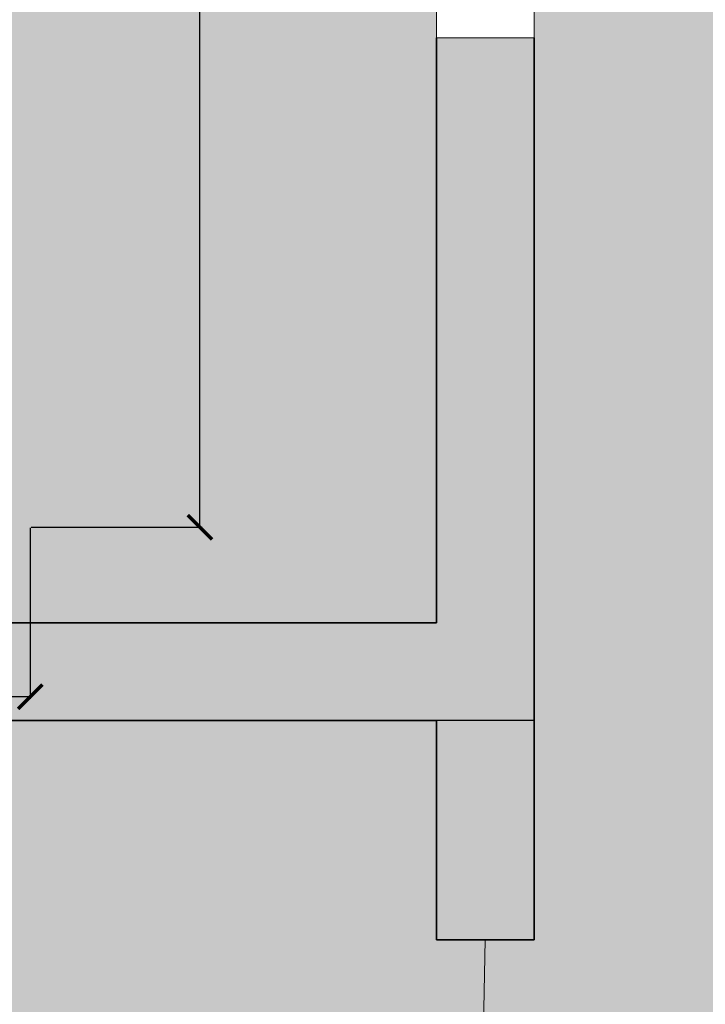
# Model space of a CAD drawing. Units: inches. Extents: x 1704 to 6393, y -157 to 1172.
# Tile 35 of 122: x 2563 to 2619, y 67 to 148. Entities that reach past the tile are written whole.
import ezdxf

# ---------------------------------------------------------------- set-up
doc = ezdxf.new("R2010")
doc.units = ezdxf.units.IN
doc.header["$MEASUREMENT"] = 0
for name, color, linetype, lineweight in [('A-ANNO-DIMS', 7, 'Continuous', 13), ('A-WALL-PATT', 7, 'Continuous', 13), ('L-HRDS', 8, 'Continuous', 18), ('L-PVMT-PATT', 8, 'Continuous', 13), ('WALLS', 7, 'Continuous', 35), ('WINDOWS', 2, 'Continuous', 18)]:
    doc.layers.add(name, color=color, linetype=linetype, lineweight=lineweight)
doc.layers.add('A-FLOR-PATT', color=7, linetype='Continuous', lineweight=13, true_color=0xf2f2f2)
doc.layers.add('L-HRDS-PATT', color=9, linetype='Continuous', lineweight=13, true_color=0xc5c1ba)
doc.styles.get("Standard").update_dxf_attribs({"font": 'arial.ttf'})
doc.dimstyles.get("Standard").update_dxf_attribs({"dimtxt": 6, "dimasz": 2, "dimexe": 0.18, "dimexo": 0.0625, "dimgap": 0.09, "dimtad": 0, "dimtih": 1, "dimtoh": 1, "dimdec": 1, "dimzin": 0, "dimdsep": 46, "dimlunit": 3, "dimtxsty": 'Standard', "dimblk": 'ARCHTICK', "dimcen": 0.09, "dimadec": 0, "dimazin": 0, "dimtfac": 1, "dimtdec": 1, "dimtofl": 0, "dimtmove": 0, "dimatfit": 3, "dimfxl": 1, "dimtolj": 1, "dimtzin": 0, "dimarcsym": 0})

# ---------------------------------------------------------------- blocks, each defined once
blk = doc.blocks.new('WIN-SLIDER-72')
for p, q in [((0, 72), (0, 0)), ((0, 72), (8, 72)), ((8, 66.251), (8, 72)), ((0, 67.227), (8, 67.227)), ((1.169, 36), (1.169, 64.3)), ((8, 7.7), (8, 64.3)), ((3.12, 37.952), (3.12, 62.348)), ((4.096, 37.952), (4.096, 62.348)), ((5.072, 37.952), (5.072, 62.348)), ((2.144, 37.952), (2.144, 42.144)), ((5.072, 36), (5.072, 7.7)), ((1.169, 9.652), (1.169, 34.048)), ((2.144, 9.652), (2.144, 34.048)), ((3.12, 9.652), (3.12, 34.048)), ((4.096, 34.048), (4.096, 29.856)), ((8, 5.749), (8, 0)), ((0, 4.773), (8, 4.773)), ((0, 0), (8, 0))]:
    blk.add_line(p, q)
for points in [[(8, 64.3), (8, 66.251), (0, 66.251), (0, 64.3)], [(5.072, 62.348), (5.072, 64.3), (3.12, 64.3), (3.12, 62.348)], [(2.144, 42.649), (1.853, 42.144), (2.436, 42.144)], [(5.072, 36), (5.072, 37.952), (3.12, 37.952), (3.12, 36)], [(3.12, 34.048), (3.12, 36), (1.169, 36), (1.169, 34.048)], [(4.096, 29.351), (3.804, 29.856), (4.388, 29.856)], [(3.12, 7.7), (3.12, 9.652), (1.169, 9.652), (1.169, 7.7)], [(8, 7.7), (8, 5.749), (0, 5.749), (0, 7.7)]]:
    blk.add_lwpolyline(points, close=True)
blk = doc.blocks.new('_ArchTick')
at = {"color": 0, "linetype": 'ByBlock', "const_width": 0.15}
blk.add_lwpolyline([(-0.5, -0.5), (0.5, 0.5)], dxfattribs=at)
blk = doc.blocks.new('*D64')
at = {"layer": 'A-ANNO-DIMS', "color": 0, "lineweight": -2, "transparency": 16777216}
for p, q in [((2564.089, 198.786), (2578.115, 198.786)), ((2577.935, 198.786), (2577.935, 155.58)), ((2577.935, 106.063), (2577.935, 149.269)), ((2564.089, 106.063), (2578.115, 106.063))]:
    blk.add_line(p, q, dxfattribs=at)
at = {"layer": 'Defpoints', "color": 0, "lineweight": -3, "transparency": 16777216}
for p in [(2564.026, 198.786), (2564.026, 106.063), (2577.935, 106.063)]:
    blk.add_point(p, dxfattribs=at)
at = {"layer": 'A-ANNO-DIMS', "color": 0, "lineweight": -2, "transparency": 16777216, "xscale": 2, "yscale": 2, "zscale": 2}
for p, rotation in [((2577.935, 198.786), 90), ((2577.935, 106.063), 270)]:
    blk.add_blockref('_ArchTick', p, dxfattribs=dict(at, rotation=rotation))
at = {"layer": 'A-ANNO-DIMS', "color": 0, "transparency": 16777216, "insert": (2577.935, 152.424), "char_height": 6, "attachment_point": 5}
blk.add_mtext('\\A1;BED 93', dxfattribs=at)
blk = doc.blocks.new('*D65')
at = {"layer": 'A-ANNO-DIMS', "color": 0, "lineweight": -2, "transparency": 16777216}
for p, q in [((2491.351, 106), (2491.351, 91.974)), ((2564.026, 106), (2564.026, 91.974)), ((2491.351, 92.154), (2523.326, 92.154)), ((2564.026, 92.154), (2532.051, 92.154))]:
    blk.add_line(p, q, dxfattribs=at)
at = {"layer": 'Defpoints', "color": 0, "lineweight": -3, "transparency": 16777216}
for p in [(2491.351, 106.063), (2564.026, 106.063), (2491.351, 92.154)]:
    blk.add_point(p, dxfattribs=at)
at = {"layer": 'A-ANNO-DIMS', "color": 0, "lineweight": -2, "transparency": 16777216, "xscale": 2, "yscale": 2, "zscale": 2, "rotation": 180}
blk.add_blockref('_ArchTick', (2491.351, 92.154), dxfattribs=at)
at = {"layer": 'A-ANNO-DIMS', "color": 0, "lineweight": -2, "transparency": 16777216, "xscale": 2, "yscale": 2, "zscale": 2}
blk.add_blockref('_ArchTick', (2564.026, 92.154), dxfattribs=at)
at = {"layer": 'A-ANNO-DIMS', "color": 0, "transparency": 16777216, "insert": (2527.689, 92.154), "char_height": 6, "attachment_point": 5}
blk.add_mtext('\\A1;73', dxfattribs=at)
blk = doc.blocks.new('*D93')
at = {"layer": 'A-ANNO-DIMS', "color": 0, "lineweight": -2, "transparency": 16777216}
for p, q in [((2605.286, 895.213), (1829.698, 895.213)), ((1829.878, 895.213), (1829.878, 495.866)), ((1829.878, 90.213), (1829.878, 489.56)), ((2605.286, 90.213), (1829.698, 90.213))]:
    blk.add_line(p, q, dxfattribs=at)
at = {"layer": 'Defpoints', "color": 0, "lineweight": -3, "transparency": 16777216}
for p in [(2605.349, 895.213), (1829.878, 90.213), (2605.349, 90.213)]:
    blk.add_point(p, dxfattribs=at)
at = {"layer": 'A-ANNO-DIMS', "color": 0, "lineweight": -2, "transparency": 16777216, "xscale": 2, "yscale": 2, "zscale": 2}
for p, rotation in [((1829.878, 895.213), 90), ((1829.878, 90.213), 270)]:
    blk.add_blockref('_ArchTick', p, dxfattribs=dict(at, rotation=rotation))
at = {"layer": 'A-ANNO-DIMS', "color": 0, "transparency": 16777216, "insert": (1829.878, 492.713), "char_height": 6, "attachment_point": 5}
blk.add_mtext('\\A1;805', dxfattribs=at)

msp = doc.modelspace()

# ---------------------------------------------------------------- hatches: boundary and pattern name
at = {"layer": 'A-FLOR-PATT', "transparency": 33554528}
h = msp.add_hatch(color=256, dxfattribs=at)
h.dxf.hatch_style = 1
h.paths.add_polyline_path([(2325.349, 863.213), (2325.349, 887.213), (2263.349, 887.213), (2167.349, 887.213), (2081.349, 887.213), (2081.349, 719.213), (2277.349, 719.213), (2277.349, 711.213), (2277.349, 372.213), (2349.349, 372.213), (2381.349, 372.213), (2381.349, 364.213), (2353.349, 364.213), (2353.349, 270.213), (2381.349, 270.213), (2381.349, 266.213), (2357.349, 266.213), (2357.349, 98.213), (2381.349, 98.213), (2385.181, 98.213), (2386.482, 98.213), (2424.215, 98.213), (2425.516, 98.213), (2429.349, 98.213), (2597.349, 98.213), (2597.349, 146.213), (2597.349, 218.213), (2597.349, 266.213), (2423.349, 266.213), (2423.349, 270.213), (2473.349, 270.213), (2473.349, 294.213), (2477.349, 294.213), (2477.349, 270.213), (2547.349, 270.213), (2547.349, 364.213), (2477.349, 364.213), (2477.349, 318.213), (2473.349, 318.213), (2473.349, 364.213), (2423.349, 364.213), (2423.349, 372.213), (2469.349, 372.213), (2469.349, 459.213), (2469.349, 538.213), (2350.349, 538.213), (2350.349, 565.713), (2358.349, 565.713), (2358.349, 545.213), (2420.349, 545.213), (2420.349, 610.213), (2358.349, 610.213), (2358.349, 589.713), (2350.349, 589.713), (2350.349, 615.213), (2425.349, 615.213), (2425.349, 607.213), (2425.349, 546.213), (2469.349, 546.213), (2514.349, 546.213), (2514.349, 607.213), (2449.349, 607.213), (2449.349, 615.213), (2451.738, 615.213), (2451.738, 659.213), (2427.738, 659.213), (2427.738, 665.213), (2367.738, 665.213), (2367.738, 667.213), (2367.738, 711.213), (2325.349, 711.213), (2325.349, 719.213), (2325.349, 755.213), (2325.349, 763.213)])
h.paths.add_polyline_path([(2233.858, 822.533, -0.187247), (2233.858, 809.14), (2231.697, 808.804, 0.084893), (2233.131, 814.486), (2230.424, 814.486, -0.104258), (2228.553, 808.313), (2217.751, 807.156, -0.222222), (2217.751, 824.517), (2228.553, 823.359, -0.104258), (2230.424, 817.186), (2233.131, 817.186, 0.084893), (2231.697, 822.868)], flags=16)
h.paths.add_polyline_path([(2213.621, 833.197), (2213.621, 798.475), (2156.048, 798.475), (2156.048, 833.197)], flags=16)
h.paths.add_polyline_path([(2203.932, 848.099), (2205.089, 837.296, -0.222222), (2187.728, 837.296), (2188.885, 848.099, -0.104258), (2195.058, 849.969), (2195.058, 852.676, 0.084893), (2189.377, 851.242), (2189.712, 853.404, -0.187247), (2203.105, 853.404), (2203.44, 851.242, 0.084893), (2197.759, 852.676), (2197.759, 849.969, -0.104258)], flags=16)
h.paths.add_polyline_path([(2181.941, 837.296, -0.222222), (2164.58, 837.296), (2165.737, 848.099, -0.104258), (2171.91, 849.969), (2171.91, 852.676, 0.084893), (2166.229, 851.242), (2166.564, 853.404, -0.187247), (2179.957, 853.404), (2180.292, 851.242, 0.084893), (2174.611, 852.676), (2174.611, 849.969, -0.104258), (2180.784, 848.099)], flags=16)
h.paths.add_polyline_path([(2205.089, 794.376), (2203.932, 783.574, -0.104258), (2197.759, 781.703), (2197.759, 778.996, 0.084893), (2203.44, 780.43), (2203.105, 778.269, -0.187247), (2189.712, 778.269), (2189.377, 780.43, 0.084893), (2195.058, 778.996), (2195.058, 781.703, -0.104258), (2188.885, 783.574), (2187.728, 794.376, -0.222222)], flags=16)
h.paths.add_polyline_path([(2181.941, 794.376), (2180.784, 783.574, -0.104258), (2174.611, 781.703), (2174.611, 778.996, 0.084893), (2180.292, 780.43), (2179.957, 778.269, -0.187247), (2166.564, 778.269), (2166.229, 780.43, 0.084893), (2171.91, 778.996), (2171.91, 781.703, -0.104258), (2165.737, 783.574), (2164.58, 794.376, -0.222222)], flags=16)
h.paths.add_polyline_path([(2151.918, 807.156), (2141.116, 808.313, -0.104258), (2139.245, 814.486), (2136.539, 814.486, 0.084893), (2137.972, 808.804), (2135.811, 809.14, -0.187247), (2135.811, 822.533), (2137.972, 822.868, 0.084893), (2136.539, 817.186), (2139.245, 817.186, -0.104258), (2141.116, 823.359), (2151.918, 824.517, -0.222222)], flags=16)
h.paths.add_polyline_path([(2357.868, 363.41), (2358.814, 363.41, 0.75376)], flags=16)
h.paths.add_polyline_path([(2372.241, 363.117), (2372.248, 363.117), (2372.248, 363.343), (2371.302, 363.343), (2371.302, 363.139, -1.360391)], flags=16)
h.paths.add_polyline_path([(2371.309, 272.716), (2371.302, 272.716), (2371.302, 272.49), (2372.248, 272.49), (2372.248, 272.693, -1.360391)], flags=16)
h.paths.add_polyline_path([(2357.875, 272.716), (2357.868, 272.716), (2357.868, 272.49), (2358.814, 272.49), (2358.814, 272.693, -1.360391)], flags=16)
h.paths.add_polyline_path([(2353.769, 363.074), (2376.347, 363.074), (2376.347, 272.759), (2353.769, 272.759)], flags=16)
h.paths.add_polyline_path([(2354.772, 362.07), (2375.344, 362.07), (2375.344, 273.762), (2354.772, 273.762)], flags=0)
h.paths.add_polyline_path([(2357.868, 363.343), (2358.814, 363.343), (2358.814, 363.117), (2357.868, 363.117)], flags=16)
h.paths.add_polyline_path([(2359.288, 359.184), (2359.288, 360.063), (2370.828, 360.063), (2370.828, 359.184), (2374.332, 359.184), (2374.332, 358.464), (2372.835, 358.464), (2372.835, 357.541), (2374.332, 357.541), (2374.332, 356.82), (2372.835, 356.82), (2372.835, 355.898), (2374.332, 355.898), (2374.332, 355.177), (2372.835, 355.177), (2372.835, 354.254), (2374.332, 354.254), (2374.332, 353.534), (2372.835, 353.534), (2372.835, 352.611), (2374.332, 352.611), (2374.332, 351.89), (2372.835, 351.89), (2372.835, 350.968), (2374.332, 350.968), (2374.332, 350.247), (2372.835, 350.247), (2372.835, 349.324), (2374.332, 349.324), (2374.332, 348.604), (2372.835, 348.604), (2372.835, 347.681), (2374.332, 347.681), (2374.332, 346.96), (2372.835, 346.96), (2372.835, 346.038), (2374.332, 346.038), (2374.332, 345.317), (2372.835, 345.317), (2372.835, 344.395), (2374.332, 344.395), (2374.332, 343.674), (2372.835, 343.674), (2372.835, 342.751), (2374.332, 342.751), (2374.332, 342.03), (2372.835, 342.03), (2372.835, 341.108), (2374.332, 341.108), (2374.332, 340.387), (2372.835, 340.387), (2372.835, 339.465), (2374.332, 339.465), (2374.332, 338.744), (2372.835, 338.744), (2372.835, 337.821), (2374.332, 337.821), (2374.332, 337.1), (2372.835, 337.1), (2372.835, 336.178), (2374.332, 336.178), (2374.332, 335.457), (2372.835, 335.457), (2372.835, 334.535), (2374.332, 334.535), (2374.332, 333.814), (2372.835, 333.814), (2372.835, 332.891), (2374.332, 332.891), (2374.332, 332.171), (2372.835, 332.171), (2372.835, 331.248), (2374.332, 331.248), (2374.332, 330.527), (2372.835, 330.527), (2372.835, 329.605), (2374.332, 329.605), (2374.332, 328.884), (2372.835, 328.884), (2372.835, 327.961), (2374.332, 327.961), (2374.332, 327.241), (2372.835, 327.241), (2372.835, 326.318), (2374.332, 326.318), (2374.332, 325.597), (2372.835, 325.597), (2372.835, 324.675), (2374.332, 324.675), (2374.332, 323.954), (2372.835, 323.954), (2372.835, 323.031), (2374.332, 323.031), (2374.332, 322.311), (2372.835, 322.311), (2372.835, 321.388), (2374.332, 321.388), (2374.332, 320.667), (2372.835, 320.667), (2372.835, 319.745), (2374.332, 319.745), (2374.332, 319.024), (2372.835, 319.024), (2372.835, 318.102), (2374.332, 318.102), (2374.332, 317.381), (2372.835, 317.381), (2372.835, 316.458), (2374.332, 316.458), (2374.332, 315.737), (2372.835, 315.737), (2372.835, 314.815), (2374.332, 314.815), (2374.332, 314.094), (2372.835, 314.094), (2372.835, 313.172), (2374.332, 313.172), (2374.332, 312.451), (2372.835, 312.451), (2372.835, 311.528), (2374.332, 311.528), (2374.332, 310.807), (2372.835, 310.807), (2372.835, 309.885), (2374.332, 309.885), (2374.332, 309.164), (2372.835, 309.164), (2372.835, 308.242), (2374.332, 308.242), (2374.332, 307.521), (2372.835, 307.521), (2372.835, 306.598), (2374.332, 306.598), (2374.332, 305.878), (2372.835, 305.878), (2372.835, 304.955), (2374.332, 304.955), (2374.332, 304.234), (2372.835, 304.234), (2372.835, 303.312), (2374.332, 303.312), (2374.332, 302.591), (2372.835, 302.591), (2372.835, 301.668), (2374.332, 301.668), (2374.332, 300.948), (2372.835, 300.948), (2372.835, 300.025), (2374.332, 300.025), (2374.332, 299.304), (2372.835, 299.304), (2372.835, 298.382), (2374.332, 298.382), (2374.332, 297.661), (2372.835, 297.661), (2372.835, 296.738), (2374.332, 296.738), (2374.332, 296.018), (2372.835, 296.018), (2372.835, 295.095), (2374.332, 295.095), (2374.332, 294.374), (2372.835, 294.374), (2372.835, 293.452), (2374.332, 293.452), (2374.332, 292.731), (2372.835, 292.731), (2372.835, 291.809), (2374.332, 291.809), (2374.332, 291.088), (2372.835, 291.088), (2372.835, 290.165), (2374.332, 290.165), (2374.332, 289.444), (2372.835, 289.444), (2372.835, 288.522), (2374.332, 288.522), (2374.332, 287.801), (2372.835, 287.801), (2372.835, 286.879), (2374.332, 286.879), (2374.332, 286.158), (2372.835, 286.158), (2372.835, 285.235), (2374.332, 285.235), (2374.332, 284.514), (2372.835, 284.514), (2372.835, 283.592), (2374.332, 283.592), (2374.332, 282.871), (2372.835, 282.871), (2372.835, 281.949), (2374.332, 281.949), (2374.332, 281.228), (2372.835, 281.228), (2372.835, 280.305), (2374.332, 280.305), (2374.332, 279.585), (2372.835, 279.585), (2372.835, 278.662), (2374.332, 278.662), (2374.332, 277.941), (2372.835, 277.941), (2372.835, 277.019), (2374.332, 277.019), (2374.332, 276.298), (2370.828, 276.298), (2370.828, 275.769), (2359.288, 275.769), (2359.288, 276.298), (2355.784, 276.298), (2355.784, 277.019), (2357.281, 277.019), (2357.281, 277.941), (2355.784, 277.941), (2355.784, 278.662), (2357.281, 278.662), (2357.281, 279.585), (2355.784, 279.585), (2355.784, 280.305), (2357.281, 280.305), (2357.281, 281.228), (2355.784, 281.228), (2355.784, 281.949), (2357.281, 281.949), (2357.281, 282.871), (2355.784, 282.871), (2355.784, 283.592), (2357.281, 283.592), (2357.281, 284.514), (2355.784, 284.514), (2355.784, 285.235), (2357.281, 285.235), (2357.281, 286.158), (2355.784, 286.158), (2355.784, 286.879), (2357.281, 286.879), (2357.281, 287.801), (2355.784, 287.801), (2355.784, 288.522), (2357.281, 288.522), (2357.281, 289.444), (2355.784, 289.444), (2355.784, 290.165), (2357.281, 290.165), (2357.281, 291.088), (2355.784, 291.088), (2355.784, 291.809), (2357.281, 291.809), (2357.281, 292.731), (2355.784, 292.731), (2355.784, 293.452), (2357.281, 293.452), (2357.281, 294.374), (2355.784, 294.374), (2355.784, 295.095), (2357.281, 295.095), (2357.281, 296.018), (2355.784, 296.018), (2355.784, 296.738), (2357.281, 296.738), (2357.281, 297.661), (2355.784, 297.661), (2355.784, 298.382), (2357.281, 298.382), (2357.281, 299.304), (2355.784, 299.304), (2355.784, 300.025), (2357.281, 300.025), (2357.281, 300.948), (2355.784, 300.948), (2355.784, 301.668), (2357.281, 301.668), (2357.281, 302.591), (2355.784, 302.591), (2355.784, 303.312), (2357.281, 303.312), (2357.281, 304.234), (2355.784, 304.234), (2355.784, 304.955), (2357.281, 304.955), (2357.281, 305.878), (2355.784, 305.878), (2355.784, 306.598), (2357.281, 306.598), (2357.281, 307.521), (2355.784, 307.521), (2355.784, 308.242), (2357.281, 308.242), (2357.281, 309.164), (2355.784, 309.164), (2355.784, 309.885), (2357.281, 309.885), (2357.281, 310.807), (2355.784, 310.807), (2355.784, 311.528), (2357.281, 311.528), (2357.281, 312.451), (2355.784, 312.451), (2355.784, 313.172), (2357.281, 313.172), (2357.281, 314.094), (2355.784, 314.094), (2355.784, 314.815), (2357.281, 314.815), (2357.281, 315.737), (2355.784, 315.737), (2355.784, 316.458), (2357.281, 316.458), (2357.281, 317.381), (2355.784, 317.381), (2355.784, 318.102), (2357.281, 318.102), (2357.281, 319.024), (2355.784, 319.024), (2355.784, 319.745), (2357.281, 319.745), (2357.281, 320.667), (2355.784, 320.667), (2355.784, 321.388), (2357.281, 321.388), (2357.281, 322.311), (2355.784, 322.311), (2355.784, 323.031), (2357.281, 323.031), (2357.281, 323.954), (2355.784, 323.954), (2355.784, 324.675), (2357.281, 324.675), (2357.281, 325.597), (2355.784, 325.597), (2355.784, 326.318), (2357.281, 326.318), (2357.281, 327.241), (2355.784, 327.241), (2355.784, 327.961), (2357.281, 327.961), (2357.281, 328.884), (2355.784, 328.884), (2355.784, 329.605), (2357.281, 329.605), (2357.281, 330.527), (2355.784, 330.527), (2355.784, 331.248), (2357.281, 331.248), (2357.281, 332.171), (2355.784, 332.171), (2355.784, 332.891), (2357.281, 332.891), (2357.281, 333.814), (2355.784, 333.814), (2355.784, 334.535), (2357.281, 334.535), (2357.281, 335.457), (2355.784, 335.457), (2355.784, 336.178), (2357.281, 336.178), (2357.281, 337.1), (2355.784, 337.1), (2355.784, 337.821), (2357.281, 337.821), (2357.281, 338.744), (2355.784, 338.744), (2355.784, 339.465), (2357.281, 339.465), (2357.281, 340.387), (2355.784, 340.387), (2355.784, 341.108), (2357.281, 341.108), (2357.281, 342.03), (2355.784, 342.03), (2355.784, 342.751), (2357.281, 342.751), (2357.281, 343.674), (2355.784, 343.674), (2355.784, 344.395), (2357.281, 344.395), (2357.281, 345.317), (2355.784, 345.317), (2355.784, 346.038), (2357.281, 346.038), (2357.281, 346.96), (2355.784, 346.96), (2355.784, 347.681), (2357.281, 347.681), (2357.281, 348.604), (2355.784, 348.604), (2355.784, 349.324), (2357.281, 349.324), (2357.281, 350.247), (2355.784, 350.247), (2355.784, 350.968), (2357.281, 350.968), (2357.281, 351.89), (2355.784, 351.89), (2355.784, 352.611), (2357.281, 352.611), (2357.281, 353.534), (2355.784, 353.534), (2355.784, 354.254), (2357.281, 354.254), (2357.281, 355.177), (2355.784, 355.177), (2355.784, 355.898), (2357.281, 355.898), (2357.281, 356.82), (2355.784, 356.82), (2355.784, 357.541), (2357.281, 357.541), (2357.281, 358.464), (2355.784, 358.464), (2355.784, 359.184)], flags=0)
at = {"layer": 'A-WALL-PATT', "transparency": 33554643}
h = msp.add_hatch(color=256, dxfattribs=at)
h.dxf.hatch_style = 1
h.paths.add_polyline_path([(2167.349, 895.213), (2073.349, 895.213), (2073.349, 887.213), (2081.349, 887.213), (2167.349, 887.213)])
h.paths.add_polyline_path([(2465.349, 895.213), (2273.349, 895.213), (2273.349, 903.213), (2263.349, 903.213), (2263.349, 895.213), (2263.349, 887.213), (2325.349, 887.213), (2325.349, 863.213), (2333.349, 863.213), (2333.349, 887.213), (2465.349, 887.213)])
h.paths.add_polyline_path([(2533.349, 895.213), (2513.349, 895.213), (2513.349, 887.213), (2513.349, 861.213), (2517.349, 861.213), (2517.349, 887.213), (2533.349, 887.213)])
h.paths.add_polyline_path([(2605.349, 895.213), (2581.349, 895.213), (2581.349, 887.213), (2597.349, 887.213), (2597.349, 854.213), (2605.349, 854.213)])
h.paths.add_polyline_path([(2605.349, 752.213), (2629.349, 752.213), (2629.349, 716.213), (2605.349, 716.213), (2605.349, 712.213), (2719.349, 712.213), (2719.349, 716.213), (2631.349, 716.213), (2631.349, 754.213), (2605.349, 754.213), (2605.349, 794.213), (2597.349, 794.213), (2597.349, 787.213), (2517.349, 787.213), (2517.349, 813.213), (2513.349, 813.213), (2513.349, 783.213), (2517.349, 783.213), (2597.349, 783.213), (2597.349, 719.213), (2517.349, 719.213), (2517.349, 753.213), (2513.349, 753.213), (2513.349, 719.213), (2365.349, 719.213), (2365.349, 763.213), (2325.349, 763.213), (2325.349, 755.213), (2357.349, 755.213), (2357.349, 719.213), (2325.349, 719.213), (2325.349, 711.213), (2547.349, 711.213), (2547.349, 615.213), (2449.349, 615.213), (2449.349, 607.213), (2514.349, 607.213), (2514.349, 546.213), (2439.349, 546.213), (2425.349, 546.213), (2425.349, 607.213), (2425.349, 615.213), (2350.349, 615.213), (2350.349, 589.713), (2358.349, 589.713), (2358.349, 610.213), (2420.349, 610.213), (2420.349, 545.213), (2358.349, 545.213), (2358.349, 565.713), (2350.349, 565.713), (2350.349, 538.213), (2469.349, 538.213), (2469.349, 459.213), (2469.349, 372.213), (2423.349, 372.213), (2423.349, 364.213), (2473.349, 364.213), (2473.349, 318.213), (2477.349, 318.213), (2477.349, 364.213), (2547.349, 364.213), (2547.349, 352.213), (2549.349, 352.213), (2549.349, 364.213), (2597.349, 364.213), (2597.349, 328.213), (2549.349, 328.213), (2547.349, 328.213), (2547.349, 326.213), (2549.349, 326.213), (2597.349, 326.213), (2605.349, 326.213), (2605.349, 377.057), (2597.349, 377.057), (2597.349, 372.213), (2477.349, 372.213), (2477.349, 451.213), (2597.349, 451.213), (2605.349, 451.213), (2605.349, 459.213), (2597.349, 459.213), (2477.349, 459.213), (2477.349, 538.213), (2597.349, 538.213), (2597.349, 495.213), (2605.349, 495.213), (2605.349, 512.213), (2631.349, 512.213), (2631.349, 568.213), (2605.349, 568.213), (2605.349, 577.213), (2597.349, 577.213), (2597.349, 542.213), (2518.349, 542.213), (2518.349, 607.213), (2532.349, 607.213), (2605.349, 607.213), (2605.349, 615.213), (2597.349, 615.213), (2551.349, 615.213), (2551.349, 711.213), (2597.349, 711.213), (2597.349, 645.213), (2605.349, 645.213), (2605.349, 712.213), (2605.349, 716.213)])
h.paths.add_polyline_path([(2605.349, 566.213), (2629.349, 566.213), (2629.349, 514.213), (2605.349, 514.213)], flags=16)
h.paths.add_polyline_path([(2381.349, 372.213), (2349.349, 372.213), (2349.349, 202.213), (2337.349, 202.213), (2337.349, 194.213), (2349.349, 194.213), (2349.349, 90.213), (2349.349, 72.213), (2357.349, 72.213), (2357.349, 90.213), (2381.349, 90.213), (2381.349, 98.213), (2357.349, 98.213), (2357.349, 266.213), (2381.349, 266.213), (2381.349, 270.213), (2353.349, 270.213), (2353.349, 364.213), (2381.349, 364.213)])
h.paths.add_polyline_path([(2605.349, 302.213), (2597.349, 302.213), (2597.349, 270.213), (2477.349, 270.213), (2477.349, 294.213), (2473.349, 294.213), (2473.349, 270.213), (2423.349, 270.213), (2423.349, 266.213), (2597.349, 266.213), (2597.349, 218.213), (2605.349, 218.213)])
h.paths.add_polyline_path([(2605.349, 146.213), (2597.349, 146.213), (2597.349, 98.213), (2429.349, 98.213), (2429.349, 90.213), (2597.349, 90.213), (2597.349, 72.213), (2605.349, 72.213), (2605.349, 90.213)])
h.paths.add_polyline_path([(2225.349, 202.213), (2049.349, 202.213), (2049.349, 194.213), (2225.349, 194.213)])
h.paths.add_polyline_path([(2289.349, 202.213), (2277.349, 202.213), (2273.349, 202.213), (2269.516, 202.213), (2269.516, 194.213), (2273.349, 194.213), (2277.349, 194.213), (2289.349, 194.213)])
h.paths.add_polyline_path([(2273.349, 372.213), (2029.19, 372.213), (2029.19, 364.213), (2273.349, 364.213)])
h.paths.add_polyline_path([(2277.349, 545.213), (2213.349, 545.213), (2213.349, 573.213), (2205.349, 573.213), (2177.349, 573.213), (2177.349, 545.213), (2073.349, 545.213), (2073.349, 538.213), (2081.349, 538.213), (2277.349, 538.213)])
h.paths.add_polyline_path([(2181.349, 545.213), (2181.349, 569.213), (2205.349, 569.213), (2205.349, 545.213)], flags=16)
h.paths.add_polyline_path([(2277.349, 719.213), (2081.349, 719.213), (2073.349, 719.213), (2073.349, 711.213), (2154.575, 711.213), (2205.349, 711.213), (2205.349, 687.213), (2205.349, 629.213), (2213.349, 629.213), (2273.349, 629.213), (2273.349, 631.213), (2207.349, 631.213), (2207.349, 707.213), (2231.349, 707.213), (2231.349, 709.213), (2207.349, 709.213), (2207.349, 711.213), (2277.349, 711.213)])
at = {"layer": 'L-HRDS-PATT', "transparency": 33554539}
h = msp.add_hatch(color=256, dxfattribs=at)
h.dxf.hatch_style = 1
h.paths.add_polyline_path([(2651.217, 368.213), (2605.349, 368.213), (2605.349, 218.213), (2605.349, 212.464), (2605.349, 210.513), (2605.349, 153.913), (2605.349, 151.962), (2605.349, 146.213), (2605.349, 90.213), (2605.349, 72.213), (2601.349, 72.213), (2600.88, 50.634), (2719.349, 50.634), (2719.349, 72.213), (2711.349, 72.213), (2663.217, 72.213), (2651.217, 72.213)])
h.paths.add_polyline_path([(2711.349, 48.634), (2600.88, 48.634), (2576.88, 48.634), (2576.88, 17.658), (2711.349, 17.658)])
h.paths.add_polyline_path([(2601.349, 72.213), (2597.349, 72.213), (2597.349, 90.213), (2429.349, 90.213), (2425.516, 90.213), (2424.215, 90.213), (2386.482, 90.213), (2385.181, 90.213), (2381.349, 90.213), (2357.349, 90.213), (2357.349, 72.213), (2349.349, 72.213), (2349.349, 90.213), (2349.349, 134.213), (2277.349, 134.213), (2277.349, 50.634), (2566.88, 50.634), (2600.88, 50.634)])
h.paths.add_polyline_path([(2349.349, 146.213), (2277.349, 146.213), (2277.349, 134.213), (2349.349, 134.213)])
h.paths.add_polyline_path([(2349.349, 158.213), (2277.349, 158.213), (2277.349, 146.213), (2349.349, 146.213)])
h.paths.add_polyline_path([(2349.349, 170.213), (2277.349, 170.213), (2277.349, 158.213), (2349.349, 158.213)])
h.paths.add_polyline_path([(2349.349, 194.213), (2337.349, 194.213), (2337.349, 202.213), (2349.349, 202.213), (2349.349, 364.213), (2277.349, 364.213), (2277.349, 202.213), (2289.349, 202.213), (2289.349, 194.213), (2277.349, 194.213), (2277.349, 170.213), (2349.349, 170.213)])
at = {"layer": 'L-PVMT-PATT', "transparency": 33554643}
h = msp.add_hatch(dxfattribs=at)
h.set_pattern_fill('GRAVEL', color=256, scale=2.4)
h.set_pattern_definition([(228.0127875, (1.728, 2.4), (-19.2, -21.6), [0.3228864, -31.9658113]), (184.9697407, (1.512, 2.16), (28.8, 2.4), [0.5540832, -54.8542194]), (132.510447, (0.96, 2.112), (24, -26.4), [0.3906912, -38.6784782]), (267.273689, (0.024, 1.512), (2.4, 48), [0.5045712, -49.9525393]), (292.833654, (0, 1.008), (-12, 28.8), [0.494772, -48.9824955]), (357.273689, (0.192, 0.552), (-48, 2.4), [0.5045712, -49.9525393]), (37.6942405, (0.696, 0.528), (-31.2, -24), [0.6672696, -66.0596365]), (72.2553284, (1.224, 0.936), (16.8, 52.8), [0.6299712, -62.3671716]), (121.4295656, (1.416, 1.536), (-19.2, 31.2), [0.50628, -50.1217755]), (175.236358, (1.152, 1.968), (26.4, -2.4), [0.5779968, -28.3218302]), (222.3974378, (0.576, 2.016), (-28.8, -26.4), [0.7474752, -74.0001]), (138.814075, (2.4, 1.488), (-16.8, 14.4), [0.2551224, -25.2572276]), (171.4692344, (2.208, 1.656), (31.2, -4.8), [0.4853688, -48.0516274]), (225, (1.728, 1.728), (-3e-16, -2.4), [0.3394104, -3.0547021]), (203.19859, (1.56, 2.016), (12, 4.8), [0.1827792, -18.0950763]), (291.80141, (1.392, 1.944), (-2.4, 7.2), [0.2584872, -12.6659083]), (30.963757, (1.488, 1.704), (7.2, 4.8), [0.4198296, -13.574455]), (161.56505, (1.848, 1.92), (4.8, -2.4), [0.3035784, -7.285888]), (16.3895403, (0, 1.944), (24, 7.2), [0.42528, -42.1028284]), (70.346176, (0.408, 2.064), (-9.6, -26.4), [0.3567864, -35.3217786]), (293.19859, (1.848, 2.4), (-4.8, 12), [0.365556, -17.9122995]), (343.6104597, (1.992, 2.064), (-24, 7.2), [0.42528, -42.1028284]), (339.443955, (0, 0.456), (-12, 4.8), [0.410112, -20.095497]), (294.7751406, (0.384, 0.312), (-12, 26.4), [0.3436272, -34.0191434]), (66.80141, (1.872, 0), (4.8, 12), [0.365556, -17.9122995]), (17.3540246, (2.016, 0.336), (-31.2, -9.6), [0.4023144, -39.8290167]), (69.443955, (0.696, 0), (-4.8, -12), [0.205056, -20.300553]), (101.309932, (1.728, 0), (-2.4, 9.6), [0.122376, -12.1152708]), (165.963757, (1.704, 0.12), (7.2, -2.4), [0.494772, -9.4006815]), (186.009006, (1.224, 0.24), (24, 2.4), [0.45852, -45.3934156]), (303.690068, (1.488, 1.488), (-2.4, 4.8), [0.3461328, -8.3071903]), (353.1572266, (1.68, 1.2), (40.8, -4.8), [0.6043056, -59.8261503]), (60.945396, (2.28, 1.128), (-9.6, -16.8), [0.2470944, -24.462418]), (90, (2.4, 1.344), (-2.4, 2.4), [0.144, -2.256]), (120.256437, (1.176, 0.312), (9.6, -16.8), [0.3334176, -33.008448]), (48.0127875, (1.008, 0.6), (19.2, 21.6), [0.6457728, -31.642925]), (0, (1.44, 1.08), (2.4, 2.4), [0.624, -1.776]), (325.3048465, (2.064, 1.08), (24, -16.8), [0.3794736, -37.5678583]), (254.054604, (2.376, 0.864), (-2.4, -9.6), [0.3494448, -17.122819]), (207.6459754, (2.28, 0.528), (-45.6, -24), [0.568956, -56.326738]), (175.4260787, (1.776, 0.264), (-31.2, 2.4), [0.6019176, -59.5897762])])
h.paths.add_polyline_path([(2719.349, 368.213), (2711.349, 368.213), (2711.349, 318.481), (2663.217, 318.481), (2663.217, 368.213), (2651.217, 368.213), (2651.217, 72.213), (2663.217, 72.213), (2663.217, 137.213), (2711.349, 137.213), (2711.349, 72.213), (2663.217, 72.213), (2651.217, 72.213), (2651.217, 368.213), (2605.349, 368.213), (2605.349, 218.213), (2605.349, 212.464), (2605.349, 210.513), (2605.349, 153.913), (2605.349, 151.962), (2605.349, 146.213), (2605.349, 90.213), (2605.349, 72.213), (2601.349, 72.213), (2600.88, 50.634), (2277.349, 50.634), (2277.349, -3.787), (2719.349, -3.787)])
h.paths.add_polyline_path([(2663.217, 272.481), (2711.349, 272.481), (2711.349, 207.213), (2663.217, 207.213)], flags=16)
h.paths.add_polyline_path([(2663.217, 202.213), (2711.349, 202.213), (2711.349, 142.213), (2663.217, 142.213)], flags=16)
h.paths.add_polyline_path([(2663.217, 277.481), (2663.217, 313.481), (2711.349, 313.481), (2711.349, 277.481)], flags=16)

# ---------------------------------------------------------------- linework, layer by layer
at = {"layer": 'L-HRDS'}
msp.add_line((2601.349, 72.213), (2600.88, 50.634), dxfattribs=at)
at = {"layer": 'WALLS'}
for p, q in [((2597.349, 98.213), (2597.349, 146.213)), ((2605.349, 90.213), (2605.349, 146.213)), ((2597.349, 98.213), (2429.349, 98.213)), ((2597.349, 90.213), (2429.349, 90.213)), ((2597.349, 90.213), (2597.349, 72.213)), ((2605.349, 90.213), (2605.349, 72.213)), ((2605.349, 72.213), (2597.349, 72.213))]:
    msp.add_line(p, q, dxfattribs=at)

# ---------------------------------------------------------------- block references
at = {"layer": 'WINDOWS'}
msp.add_blockref('WIN-SLIDER-72', (2597.349, 146.213), dxfattribs=at)

# ---------------------------------------------------------------- dimensions: what is measured, and where the dimension line sits
at = {"layer": 'A-ANNO-DIMS'}
for base, p1, p2, angle, picture, middle in [((1829.878, 90.213), (2605.349, 895.213), (2605.349, 90.213), 90, '*D93', (1829.878, 492.713)), ((2491.351, 92.154), (2564.026, 106.063), (2491.351, 106.063), 180, '*D65', (2527.689, 92.154))]:
    dim = msp.add_linear_dim(base=base, p1=p1, p2=p2, angle=angle, dimstyle='Standard', override={"dimdec": 0, "dimlfac": 1, "dimrnd": 0, "dimzin": 0, "dimdsep": 46, "dimlunit": 2}, dxfattribs=at)
    dim.commit()
    dim.dimension.update_dxf_attribs({"geometry": picture, "text_midpoint": middle})
dim = msp.add_linear_dim(base=(2577.935, 106.063), p1=(2564.026, 198.786), p2=(2564.026, 106.063), angle=270, text='BED <>', dimstyle='Standard', override={"dimdec": 0, "dimlfac": 1, "dimrnd": 0, "dimzin": 0, "dimdsep": 46, "dimlunit": 2}, dxfattribs=at)
dim.commit()
dim.dimension.update_dxf_attribs({"geometry": '*D64', "text_midpoint": (2577.935, 152.424)})

doc.saveas('drawing.dxf')
